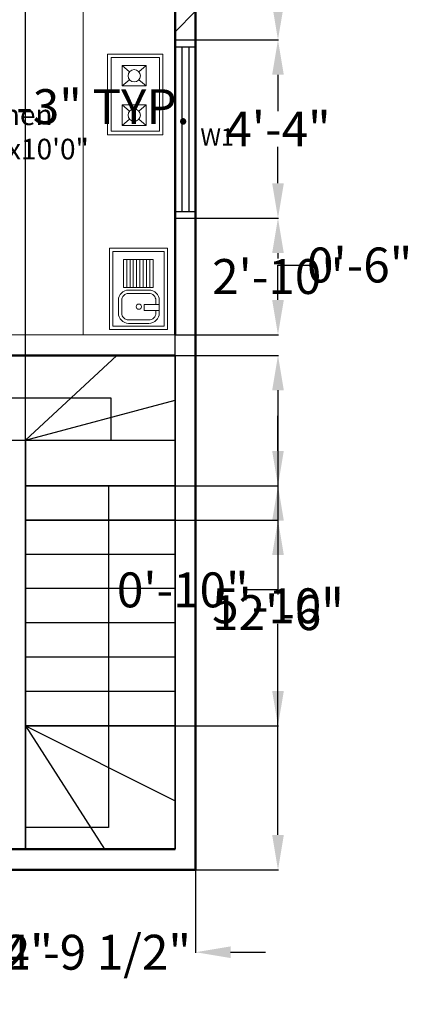
# Model space of a CAD drawing. Units: inches. Extents: x 21 to 3450, y 4 to 2137.
# Tile 13 of 14: x 3335 to 3450, y 1057 to 1344. Entities that reach past the tile are written whole.
import ezdxf

# ---------------------------------------------------------------- set-up
doc = ezdxf.new("R2010")
doc.units = ezdxf.units.IN
doc.header["$MEASUREMENT"] = 0
for name, color, linetype, lineweight in [('A-ANNO-DIMS', 2, 'Continuous', 18), ('A-ANNO-TEXT', 7, 'Continuous', 18), ('A-AREA-IDEN', 3, 'Continuous', 18), ('A-FLOR-FIXT', 9, 'Continuous', 18), ('A-FLOR-STRS', 2, 'Continuous', 25), ('A-FURN', 8, 'Continuous', 18), ('A-GLAZ', 3, 'Continuous', 25), ('A-WALL', 7, 'Continuous', 50), ('A-WALL-PATT', 8, 'Continuous', 13)]:
    doc.layers.add(name, color=color, linetype=linetype, lineweight=lineweight)
doc.styles.get("Standard").update_dxf_attribs({"font": 'arial.ttf'})
doc.dimstyles.get("Standard").update_dxf_attribs({"dimtxt": 10.18, "dimasz": 10.18, "dimexe": 0.18, "dimexo": 0.0625, "dimgap": 0.09, "dimtad": 0, "dimtih": 1, "dimtoh": 1, "dimdec": 0, "dimzin": 0, "dimdsep": 46, "dimlunit": 3, "dimtxsty": 'Standard', "dimcen": 0.09, "dimadec": 0, "dimazin": 0, "dimtfac": 1, "dimtdec": 0, "dimtofl": 0, "dimtmove": 0, "dimatfit": 3, "dimfxl": 1, "dimtolj": 1, "dimtzin": 0, "dimarcsym": 0})

# ---------------------------------------------------------------- blocks, each defined once
blk = doc.blocks.new('STOVE-BURNER')
blk.add_line((0, 5.99), (2.12, 4.17))
blk.add_lwpolyline([(0, 5.99), (0, 5.99), (6.94, 5.99), (6.94, 5.99), (6.94, 0), (6.94, 0), (0, 0), (0, 0)], close=True)
blk = doc.blocks.new('*D30')
at = {"layer": 'A-ANNO-DIMS', "color": 0, "lineweight": -2, "transparency": 16777216}
for p, q in [((3201.06, 1318.3), (3190.88, 1318.3)), ((3211.24, 1320.48), (3211.24, 1318.12)), ((3226.19, 1320.48), (3226.19, 1318.12)), ((3236.37, 1318.3), (3246.55, 1318.3))]:
    blk.add_line(p, q, dxfattribs=at)
at = {"layer": 'A-ANNO-DIMS', "color": 0, "transparency": 16777216}
for points in [[(3201.06, 1320), (3201.06, 1316.61), (3211.24, 1318.3)], [(3236.37, 1320), (3236.37, 1316.61), (3226.19, 1318.3)]]:
    blk.add_solid(points, dxfattribs=at)
at = {"layer": 'Defpoints', "color": 0, "transparency": 16777216}
for p in [(3211.24, 1320.54), (3226.19, 1320.54), (3226.19, 1318.3)]:
    blk.add_point(p, dxfattribs=at)
at = {"layer": 'A-ANNO-DIMS', "color": 0, "transparency": 16777216, "insert": (3317.86, 1318.3), "char_height": 10.18, "attachment_point": 5}
blk.add_mtext('\\A1;ARMCHAIR 1\'-3" TYP.', dxfattribs=at)
blk = doc.blocks.new('*D131')
at = {"layer": 'A-ANNO-DIMS', "color": 0, "lineweight": -2, "transparency": 16777216}
for p, q in [((3254.61, 1101.7), (3254.61, 1071.59)), ((3272.34, 1095.7), (3272.34, 1071.59)), ((3244.43, 1071.77), (3234.25, 1071.77)), ((3282.52, 1071.77), (3292.7, 1071.77))]:
    blk.add_line(p, q, dxfattribs=at)
at = {"layer": 'A-ANNO-DIMS', "color": 0, "transparency": 16777216}
for points in [[(3244.43, 1073.46), (3244.43, 1070.07), (3254.61, 1071.77)], [(3282.52, 1073.46), (3282.52, 1070.07), (3272.34, 1071.77)]]:
    blk.add_solid(points, dxfattribs=at)
at = {"layer": 'Defpoints', "color": 0, "transparency": 16777216}
for p in [(3254.61, 1101.77), (3272.34, 1095.77), (3272.34, 1071.77)]:
    blk.add_point(p, dxfattribs=at)
at = {"layer": 'A-ANNO-DIMS', "color": 0, "transparency": 16777216, "insert": (3317.7, 1071.77), "char_height": 10.18, "attachment_point": 5}
blk.add_mtext('\\A1;1\'-5 1/2"', dxfattribs=at)
blk = doc.blocks.new('*D133')
at = {"layer": 'A-ANNO-DIMS', "color": 0, "lineweight": -2, "transparency": 16777216}
for p, q in [((3329.26, 1095.7), (3329.26, 1071.59)), ((3386.61, 1095.7), (3386.61, 1071.59)), ((3319.08, 1071.77), (3308.9, 1071.77)), ((3396.79, 1071.77), (3406.97, 1071.77))]:
    blk.add_line(p, q, dxfattribs=at)
at = {"layer": 'A-ANNO-DIMS', "color": 0, "transparency": 16777216}
for points in [[(3319.08, 1073.46), (3319.08, 1070.07), (3329.26, 1071.77)], [(3396.79, 1073.46), (3396.79, 1070.07), (3386.61, 1071.77)]]:
    blk.add_solid(points, dxfattribs=at)
at = {"layer": 'Defpoints', "color": 0, "transparency": 16777216}
for p in [(3329.26, 1095.77), (3386.61, 1095.77), (3386.61, 1071.77)]:
    blk.add_point(p, dxfattribs=at)
at = {"layer": 'A-ANNO-DIMS', "color": 0, "transparency": 16777216, "insert": (3357.93, 1071.77), "char_height": 10.18, "attachment_point": 5}
blk.add_mtext('\\A1;4\'-9 1/2"', dxfattribs=at)
blk = doc.blocks.new('*D134')
at = {"layer": 'A-ANNO-DIMS', "color": 0, "lineweight": -2, "transparency": 16777216}
for p, q in [((3380.67, 1245.77), (3410.79, 1245.77)), ((3410.61, 1235.59), (3410.61, 1176.05)), ((3410.61, 1105.95), (3410.61, 1165.48)), ((3386.67, 1095.77), (3410.79, 1095.77))]:
    blk.add_line(p, q, dxfattribs=at)
at = {"layer": 'A-ANNO-DIMS', "color": 0, "transparency": 16777216}
for points in [[(3408.91, 1235.59), (3412.31, 1235.59), (3410.61, 1245.77)], [(3408.91, 1105.95), (3412.31, 1105.95), (3410.61, 1095.77)]]:
    blk.add_solid(points, dxfattribs=at)
at = {"layer": 'Defpoints', "color": 0, "transparency": 16777216}
for p in [(3380.61, 1245.77), (3410.61, 1245.77), (3386.61, 1095.77)]:
    blk.add_point(p, dxfattribs=at)
at = {"layer": 'A-ANNO-DIMS', "color": 0, "transparency": 16777216, "insert": (3410.61, 1170.77), "char_height": 10.18, "attachment_point": 5}
blk.add_mtext('\\A1;12\'-6"', dxfattribs=at)
blk = doc.blocks.new('*D135')
at = {"layer": 'A-ANNO-DIMS', "color": 0, "lineweight": -2, "transparency": 16777216}
for p, q in [((3410.61, 1261.95), (3410.61, 1272.13)), ((3410.61, 1272.13), (3420.79, 1272.13)), ((3380.67, 1251.77), (3410.79, 1251.77)), ((3380.67, 1245.77), (3410.79, 1245.77)), ((3410.61, 1235.59), (3410.61, 1225.41))]:
    blk.add_line(p, q, dxfattribs=at)
at = {"layer": 'A-ANNO-DIMS', "color": 0, "transparency": 16777216}
for points in [[(3408.91, 1261.95), (3412.31, 1261.95), (3410.61, 1251.77)], [(3408.91, 1235.59), (3412.31, 1235.59), (3410.61, 1245.77)]]:
    blk.add_solid(points, dxfattribs=at)
at = {"layer": 'Defpoints', "color": 0, "transparency": 16777216}
for p in [(3380.61, 1251.77), (3410.61, 1251.77), (3380.61, 1245.77)]:
    blk.add_point(p, dxfattribs=at)
at = {"layer": 'A-ANNO-DIMS', "color": 0, "transparency": 16777216, "insert": (3434.41, 1272.13), "char_height": 10.18, "attachment_point": 5}
blk.add_mtext('\\A1;0\'-6"', dxfattribs=at)
blk = doc.blocks.new('*D136')
at = {"layer": 'A-ANNO-DIMS', "color": 0, "lineweight": -2, "transparency": 16777216}
for p, q in [((3386.67, 1285.77), (3410.79, 1285.77)), ((3410.61, 1275.59), (3410.61, 1274.05)), ((3410.61, 1261.95), (3410.61, 1263.48)), ((3380.67, 1251.77), (3410.79, 1251.77))]:
    blk.add_line(p, q, dxfattribs=at)
at = {"layer": 'A-ANNO-DIMS', "color": 0, "transparency": 16777216}
for points in [[(3408.91, 1275.59), (3412.31, 1275.59), (3410.61, 1285.77)], [(3408.91, 1261.95), (3412.31, 1261.95), (3410.61, 1251.77)]]:
    blk.add_solid(points, dxfattribs=at)
at = {"layer": 'Defpoints', "color": 0, "transparency": 16777216}
for p in [(3386.61, 1285.77), (3410.61, 1285.77), (3380.61, 1251.77)]:
    blk.add_point(p, dxfattribs=at)
at = {"layer": 'A-ANNO-DIMS', "color": 0, "transparency": 16777216, "insert": (3410.61, 1268.77), "char_height": 10.18, "attachment_point": 5}
blk.add_mtext('\\A1;2\'-10"', dxfattribs=at)
blk = doc.blocks.new('*D137')
at = {"layer": 'A-ANNO-DIMS', "color": 0, "lineweight": -2, "transparency": 16777216}
for p, q in [((3386.67, 1337.77), (3410.79, 1337.77)), ((3410.61, 1327.59), (3410.61, 1316.95)), ((3410.61, 1295.95), (3410.61, 1306.59)), ((3386.67, 1285.77), (3410.79, 1285.77))]:
    blk.add_line(p, q, dxfattribs=at)
at = {"layer": 'A-ANNO-DIMS', "color": 0, "transparency": 16777216}
for points in [[(3408.91, 1327.59), (3412.31, 1327.59), (3410.61, 1337.77)], [(3408.91, 1295.95), (3412.31, 1295.95), (3410.61, 1285.77)]]:
    blk.add_solid(points, dxfattribs=at)
at = {"layer": 'Defpoints', "color": 0, "transparency": 16777216}
for p in [(3386.61, 1337.77), (3410.61, 1337.77), (3386.61, 1285.77)]:
    blk.add_point(p, dxfattribs=at)
at = {"layer": 'A-ANNO-DIMS', "color": 0, "transparency": 16777216, "insert": (3410.61, 1311.77), "char_height": 10.18, "attachment_point": 5}
blk.add_mtext('\\A1;4\'-4"', dxfattribs=at)
blk = doc.blocks.new('*D138')
at = {"layer": 'A-ANNO-DIMS', "color": 0, "lineweight": -2, "transparency": 16777216}
for p, q in [((3380.67, 1371.77), (3410.79, 1371.77)), ((3410.61, 1361.59), (3410.61, 1360.05)), ((3410.61, 1347.95), (3410.61, 1349.48)), ((3386.67, 1337.77), (3410.79, 1337.77))]:
    blk.add_line(p, q, dxfattribs=at)
at = {"layer": 'A-ANNO-DIMS', "color": 0, "transparency": 16777216}
for points in [[(3408.91, 1361.59), (3412.31, 1361.59), (3410.61, 1371.77)], [(3408.91, 1347.95), (3412.31, 1347.95), (3410.61, 1337.77)]]:
    blk.add_solid(points, dxfattribs=at)
at = {"layer": 'Defpoints', "color": 0, "transparency": 16777216}
for p in [(3380.61, 1371.77), (3410.61, 1371.77), (3386.61, 1337.77)]:
    blk.add_point(p, dxfattribs=at)
at = {"layer": 'A-ANNO-DIMS', "color": 0, "transparency": 16777216, "insert": (3410.61, 1354.77), "char_height": 10.18, "attachment_point": 5}
blk.add_mtext('\\A1;2\'-10"', dxfattribs=at)
blk = doc.blocks.new('*D148')
at = {"layer": 'A-ANNO-DIMS', "color": 0, "lineweight": -2, "transparency": 16777216}
for p, q in [((3337.06, 1101.83), (3337.06, 1548.11)), ((3347.24, 1547.93), (3370.43, 1547.93)), ((3380.61, 1101.83), (3380.61, 1548.11)), ((3380.61, 1547.93), (3390.79, 1547.93))]:
    blk.add_line(p, q, dxfattribs=at)
at = {"layer": 'A-ANNO-DIMS', "color": 0, "transparency": 16777216}
for points in [[(3347.24, 1549.63), (3347.24, 1546.23), (3337.06, 1547.93)], [(3370.43, 1549.63), (3370.43, 1546.23), (3380.61, 1547.93)]]:
    blk.add_solid(points, dxfattribs=at)
at = {"layer": 'Defpoints', "color": 0, "transparency": 16777216}
for p in [(3380.61, 1547.93), (3337.06, 1101.77), (3380.61, 1101.77)]:
    blk.add_point(p, dxfattribs=at)
at = {"layer": 'A-ANNO-DIMS', "color": 0, "transparency": 16777216, "insert": (3416.27, 1547.93), "char_height": 10.18, "attachment_point": 5}
blk.add_mtext('\\A1;3\'-7 1/2"', dxfattribs=at)
blk = doc.blocks.new('*D149')
at = {"layer": 'A-ANNO-DIMS', "color": 0, "lineweight": -2, "transparency": 16777216}
for p, q in [((3410.61, 1217.95), (3410.61, 1228.13)), ((3337.12, 1207.77), (3410.79, 1207.77)), ((3337.12, 1197.77), (3410.79, 1197.77)), ((3410.61, 1187.59), (3410.61, 1177.41)), ((3410.61, 1177.41), (3400.43, 1177.41))]:
    blk.add_line(p, q, dxfattribs=at)
at = {"layer": 'A-ANNO-DIMS', "color": 0, "transparency": 16777216}
for points in [[(3408.91, 1217.95), (3412.31, 1217.95), (3410.61, 1207.77)], [(3408.91, 1187.59), (3412.31, 1187.59), (3410.61, 1197.77)]]:
    blk.add_solid(points, dxfattribs=at)
at = {"layer": 'Defpoints', "color": 0, "transparency": 16777216}
for p in [(3337.06, 1207.77), (3337.06, 1197.77), (3410.61, 1197.77)]:
    blk.add_point(p, dxfattribs=at)
at = {"layer": 'A-ANNO-DIMS', "color": 0, "transparency": 16777216, "insert": (3382.86, 1177.41), "char_height": 10.18, "attachment_point": 5}
blk.add_mtext('\\A1;0\'-10"', dxfattribs=at)
blk = doc.blocks.new('*D150')
at = {"layer": 'A-ANNO-DIMS', "color": 0, "lineweight": -2, "transparency": 16777216}
for p, q in [((3337.12, 1207.77), (3410.79, 1207.77)), ((3410.61, 1197.59), (3410.61, 1178.05)), ((3410.61, 1147.95), (3410.61, 1167.48)), ((3337.12, 1137.77), (3410.79, 1137.77))]:
    blk.add_line(p, q, dxfattribs=at)
at = {"layer": 'A-ANNO-DIMS', "color": 0, "transparency": 16777216}
for points in [[(3408.91, 1197.59), (3412.31, 1197.59), (3410.61, 1207.77)], [(3408.91, 1147.95), (3412.31, 1147.95), (3410.61, 1137.77)]]:
    blk.add_solid(points, dxfattribs=at)
at = {"layer": 'Defpoints', "color": 0, "transparency": 16777216}
for p in [(3337.06, 1207.77), (3337.06, 1137.77), (3410.61, 1137.77)]:
    blk.add_point(p, dxfattribs=at)
at = {"layer": 'A-ANNO-DIMS', "color": 0, "transparency": 16777216, "insert": (3410.61, 1172.77), "char_height": 10.18, "attachment_point": 5}
blk.add_mtext('\\A1;5\'-10"', dxfattribs=at)

msp = doc.modelspace()

# ---------------------------------------------------------------- hatches: boundary and pattern name
at = {"layer": 'A-WALL-PATT'}
h = msp.add_hatch(dxfattribs=at)
h.set_pattern_fill('ANSI31', color=256, scale=46)
h.set_pattern_definition([(45, (297.6833, 160.0466), (-4.065864, 4.065864), [])])
h.paths.add_polyline_path([(3281.11, 1515.77), (3146.61, 1515.77), (3146.61, 1199.77), (3152.61, 1199.77), (3152.61, 1245.77), (3152.61, 1251.77), (3152.61, 1371.77), (3152.61, 1377.77), (3152.61, 1461.77), (3176.11, 1461.77), (3176.11, 1467.77), (3152.61, 1467.77), (3152.61, 1509.77), (3227.61, 1509.77), (3233.61, 1509.77), (3281.11, 1509.77)])
h.paths.add_polyline_path([(3386.61, 1515.77), (3333.11, 1515.77), (3333.11, 1509.77), (3380.61, 1509.77), (3380.61, 1469.33, -0.065004), (3380.75, 1468.31), (3380.75, 1431.5, -0.065004), (3380.61, 1430.47), (3380.61, 1377.77), (3272.1, 1377.77), (3272.1, 1374.77), (3274.1, 1374.77), (3274.1, 1371.77), (3302.61, 1371.77), (3302.61, 1345.32), (3308.61, 1345.32), (3308.61, 1371.77), (3380.61, 1371.77), (3380.61, 1337.77), (3386.61, 1337.77)])
h.paths.add_polyline_path([(3215.61, 1248.77), (3215.61, 1251.77), (3182.61, 1251.77), (3182.61, 1333.19), (3176.61, 1333.19), (3176.61, 1251.77), (3176.61, 1245.77), (3215.61, 1245.77), (3215.61, 1246.77, -0.014283)], flags=17)
h.paths.add_polyline_path([(3177.61, 1101.77), (3152.61, 1101.77), (3152.61, 1147.77), (3146.61, 1147.77), (3146.61, 1095.77), (3177.61, 1095.77)])
h.paths.add_polyline_path([(3241.1, 1377.77), (3233.61, 1377.77), (3227.61, 1377.77), (3176.61, 1377.77), (3176.61, 1371.77), (3182.61, 1371.77), (3233.61, 1371.77), (3241.1, 1371.77)], flags=17)
h.paths.add_polyline_path([(3233.61, 1467.77), (3227.61, 1467.77), (3204.11, 1467.77), (3204.11, 1461.77), (3227.61, 1461.77), (3227.61, 1410.77), (3228.61, 1410.77, -0.017236), (3230.61, 1410.77), (3233.61, 1410.77), (3233.61, 1461.77)], flags=17)

# ---------------------------------------------------------------- linework, layer by layer
at = {"layer": 'A-FLOR-FIXT'}
for p, q in [((3353.85, 1251.77), (3353.85, 1349.33)), ((3372.18, 1330.31), (3370.07, 1328.48)), ((3365.24, 1324.32), (3367.36, 1326.14)), ((3372.18, 1324.32), (3370.07, 1326.14)), ((3372.18, 1318.82), (3370.07, 1316.99)), ((3365.24, 1312.83), (3367.36, 1314.65)), ((3372.18, 1312.83), (3370.07, 1314.65))]:
    msp.add_line(p, q, dxfattribs=at)
for points in [[(3360.97, 1333.58), (3360.97, 1333.58), (3377.06, 1333.58), (3377.06, 1333.58), (3377.06, 1310.11), (3377.06, 1310.11), (3360.97, 1310.11), (3360.97, 1310.11)], [(3361.97, 1332.58), (3376.06, 1332.58), (3376.06, 1311.11), (3361.97, 1311.11)], [(3378.4, 1277.07), (3361.52, 1277.07), (3361.52, 1253.32), (3378.4, 1253.32)], [(3377.4, 1276.07), (3377.4, 1276.07), (3362.52, 1276.07), (3362.52, 1276.07), (3362.52, 1254.32), (3362.52, 1254.32), (3377.4, 1254.32), (3377.4, 1254.32)], [(3365.56, 1273.78), (3365.56, 1273.78), (3366.52, 1273.78), (3366.52, 1273.78), (3366.52, 1265.58), (3366.52, 1265.58), (3365.56, 1265.58), (3365.56, 1265.58)], [(3366.52, 1273.78), (3366.52, 1273.78), (3367.49, 1273.78), (3367.49, 1273.78), (3367.49, 1265.58), (3367.49, 1265.58), (3366.52, 1265.58), (3366.52, 1265.58)], [(3367.49, 1273.78), (3367.49, 1273.78), (3368.45, 1273.78), (3368.45, 1273.78), (3368.45, 1265.58), (3368.45, 1265.58), (3367.49, 1265.58), (3367.49, 1265.58)], [(3368.45, 1273.78), (3368.45, 1273.78), (3369.42, 1273.78), (3369.42, 1273.78), (3369.42, 1265.58), (3369.42, 1265.58), (3368.45, 1265.58), (3368.45, 1265.58)], [(3369.42, 1273.78), (3369.42, 1273.78), (3370.38, 1273.78), (3370.38, 1273.78), (3370.38, 1265.58), (3370.38, 1265.58), (3369.42, 1265.58), (3369.42, 1265.58)], [(3370.38, 1273.78), (3370.38, 1273.78), (3371.35, 1273.78), (3371.35, 1273.78), (3371.35, 1265.58), (3371.35, 1265.58), (3370.38, 1265.58), (3370.38, 1265.58)], [(3371.35, 1273.78), (3371.35, 1273.78), (3372.32, 1273.78), (3372.32, 1273.78), (3372.32, 1265.58), (3372.32, 1265.58), (3371.35, 1265.58), (3371.35, 1265.58)], [(3372.32, 1273.78), (3372.32, 1273.78), (3373.28, 1273.78), (3373.28, 1273.78), (3373.28, 1265.58), (3373.28, 1265.58), (3372.32, 1265.58), (3372.32, 1265.58)], [(3373.28, 1273.78), (3373.28, 1273.78), (3374.25, 1273.78), (3374.25, 1273.78), (3374.25, 1265.58), (3374.25, 1265.58), (3373.28, 1265.58), (3373.28, 1265.58)], [(3376.01, 1260.63), (3376.01, 1260.63), (3371.61, 1260.63), (3371.61, 1260.63), (3371.61, 1258.82), (3371.61, 1258.82), (3376.01, 1258.82), (3376.01, 1258.82)]]:
    msp.add_lwpolyline(points, close=True, dxfattribs=at)
msp.add_lwpolyline([(3364.09, 1261.83, -0.414214), (3367.09, 1264.83), (3373.01, 1264.83, -0.414214), (3376.01, 1261.83), (3376.01, 1258.12, -0.414214), (3373.01, 1255.12), (3367.09, 1255.12, -0.414214), (3364.09, 1258.12)], format="xyb", close=True, dxfattribs=at)
msp.add_lwpolyline([(3375.01, 1258.82), (3375.01, 1258.12, -0.414214), (3373.01, 1256.12), (3367.09, 1256.12, -0.414214), (3365.09, 1258.12), (3365.09, 1261.83, -0.414214), (3367.09, 1263.83), (3373.01, 1263.83, -0.414214), (3375.01, 1261.83), (3375.01, 1260.63)], format="xyb", dxfattribs=at)
for centre, radius in [((3368.71, 1327.31), 1.79), ((3368.71, 1315.82), 1.79), ((3370.05, 1259.98), 0.767)]:
    msp.add_circle(centre, radius, dxfattribs=at)
at = {"layer": 'A-FLOR-STRS'}
for p, q in [((3337.06, 1221.07), (3337.06, 1245.77)), ((3337.06, 1221.07), (3363.67, 1245.77)), ((3380.61, 1245.77), (3380.61, 1101.77)), ((3302.61, 1233.42), (3361.91, 1233.42)), ((3337.06, 1221.07), (3380.61, 1232.74)), ((3361.91, 1233.42), (3361.91, 1221.07)), ((3302.61, 1221.07), (3337.06, 1221.07)), ((3337.06, 1221.07), (3337.06, 1101.77)), ((3337.06, 1221.07), (3380.61, 1221.07)), ((3380.61, 1207.77), (3337.06, 1207.77)), ((3361.17, 1207.77), (3361.17, 1108.09)), ((3380.61, 1197.77), (3337.06, 1197.77)), ((3380.61, 1197.77), (3337.06, 1197.77)), ((3380.61, 1187.77), (3337.06, 1187.77)), ((3380.61, 1177.77), (3337.06, 1177.77)), ((3380.61, 1167.77), (3337.06, 1167.77)), ((3380.61, 1157.77), (3337.06, 1157.77)), ((3380.61, 1147.77), (3337.06, 1147.77)), ((3380.61, 1137.77), (3337.06, 1137.77)), ((3337.06, 1137.77), (3380.61, 1115.89)), ((3337.06, 1137.77), (3360.02, 1101.77)), ((3361.17, 1108.09), (3337.06, 1108.09))]:
    msp.add_line(p, q, dxfattribs=at)
at = {"layer": 'A-FURN'}
msp.add_line((3308.61, 1251.77), (3380.61, 1251.77), dxfattribs=at)
at = {"layer": 'A-GLAZ'}
for p, q in [((3380.61, 1337.77), (3386.61, 1337.77)), ((3380.61, 1335.77), (3386.61, 1335.77)), ((3382.61, 1335.77), (3382.61, 1287.77)), ((3384.61, 1335.77), (3384.61, 1287.77)), ((3380.61, 1287.77), (3386.61, 1287.77)), ((3380.61, 1285.77), (3386.61, 1285.77))]:
    msp.add_line(p, q, dxfattribs=at)
at = {"layer": 'A-WALL'}
for p, q in [((3386.61, 1515.77), (3386.61, 1095.77)), ((3380.61, 1371.77), (3380.61, 1251.77)), ((3260.61, 1245.77), (3380.61, 1245.77)), ((3380.61, 1101.77), (3329.26, 1101.77)), ((3386.61, 1095.77), (3329.26, 1095.77))]:
    msp.add_line(p, q, dxfattribs=at)

# ---------------------------------------------------------------- block references
at = {"layer": 'A-FLOR-FIXT'}
for p in [(3365.24, 1324.32), (3365.24, 1312.83)]:
    msp.add_blockref('STOVE-BURNER', p, dxfattribs=at)

# ---------------------------------------------------------------- texts
at = {"layer": 'A-ANNO-TEXT', "insert": (3387.99, 1311.97), "char_height": 5, "attachment_point": 1}
msp.add_mtext_dynamic_manual_height_columns('W1', width=14.628, gutter_width=1, heights=[0], dxfattribs=at)
at = {"layer": 'A-AREA-IDEN', "insert": (3316.4, 1318.93), "char_height": 6, "attachment_point": 1}
msp.add_mtext_dynamic_manual_height_columns('kitchen\\P6\'0"x10\'0"', width=84.0083, gutter_width=1, heights=[0], dxfattribs=at)

# ---------------------------------------------------------------- dimensions: what is measured, and where the dimension line sits
at = {"layer": 'A-ANNO-DIMS'}
for base, p1, p2, picture, middle in [((3380.611, 1547.9292), (3337.0593, 1101.7664), (3380.611, 1101.7664), '*D148', (3416.2685, 1547.9292)), ((3272.34, 1071.77), (3254.61, 1101.77), (3272.34, 1095.77), '*D131', (3317.7, 1071.77)), ((3386.611, 1071.7664), (3329.2573, 1095.7664), (3386.611, 1095.7664), '*D133', (3357.9341, 1071.7664))]:
    dim = msp.add_linear_dim(base=base, p1=p1, p2=p2, dimstyle='Standard', override={"dimdec": 1, "dimlfac": 1, "dimrnd": 0, "dimzin": 1, "dimdsep": 46, "dimlunit": 4, "dimfrac": 2}, dxfattribs=at)
    dim.commit()
    dim.dimension.update_dxf_attribs({"geometry": picture, "text_midpoint": middle})
for base, p1, p2, picture, middle in [((3410.61, 1371.77), (3386.61, 1337.77), (3380.61, 1371.77), '*D138', (3410.61, 1354.77)), ((3410.61, 1337.77), (3386.61, 1285.77), (3386.61, 1337.77), '*D137', (3410.61, 1311.77)), ((3410.61, 1285.77), (3380.61, 1251.77), (3386.61, 1285.77), '*D136', (3410.61, 1268.77)), ((3410.61, 1251.77), (3380.61, 1245.77), (3380.61, 1251.77), '*D135', (3434.41, 1272.13)), ((3410.61, 1245.77), (3386.61, 1095.77), (3380.61, 1245.77), '*D134', (3410.61, 1170.77)), ((3410.61, 1197.77), (3337.06, 1207.77), (3337.06, 1197.77), '*D149', (3382.86, 1177.41)), ((3410.61, 1137.77), (3337.06, 1207.77), (3337.06, 1137.77), '*D150', (3410.61, 1172.77))]:
    dim = msp.add_linear_dim(base=base, p1=p1, p2=p2, angle=90, dimstyle='Standard', override={"dimdec": 1, "dimlfac": 1, "dimrnd": 0, "dimzin": 1, "dimdsep": 46, "dimlunit": 4, "dimfrac": 2}, dxfattribs=at)
    dim.commit()
    dim.dimension.update_dxf_attribs({"geometry": picture, "text_midpoint": middle})
dim = msp.add_linear_dim(base=(3226.1906, 1318.3019), p1=(3211.2391, 1320.5447), p2=(3226.1906, 1320.5447), text='ARMCHAIR <> TYP.', dimstyle='Standard', override={"dimdec": 1, "dimrnd": 0, "dimzin": 1, "dimlunit": 4, "dimfrac": 2}, dxfattribs=at)
dim.commit()
dim.dimension.update_dxf_attribs({"geometry": '*D30', "text_midpoint": (3317.8624, 1318.3019)})

doc.saveas('drawing.dxf')
